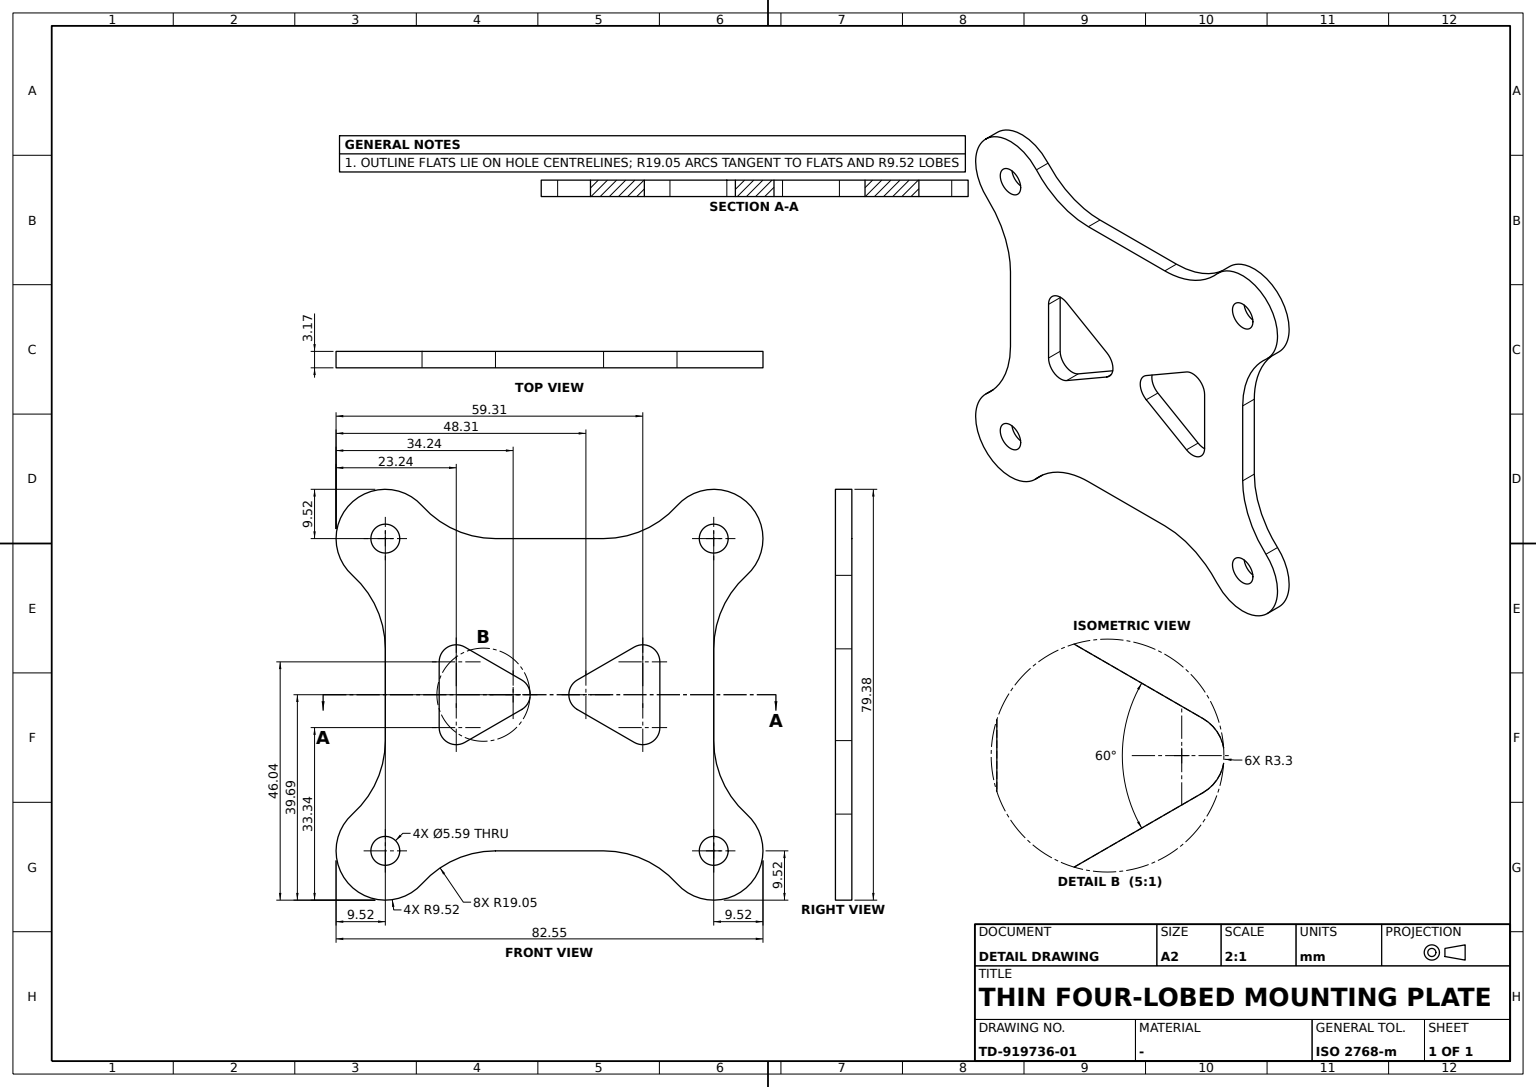
CATIA V5 part; units mm, degrees
sketch "Sketch1" plane through (0, 0, 0) normal (1, 0, 0) x (0, 1, 0)
  line L0 (31.75, 30.1625) -> (31.75, -30.1625)
  line L1 (31.75, -30.1625) -> (-31.75, -30.1625)
  line L2 (-31.75, -30.1625) -> (-31.75, 30.1625)
  line L3 (-31.75, 30.1625) -> (31.75, 30.1625)
  dimension "length L3" = 63.5
  dimension "length L2" = 60.325
  constraint vertical L0 y-axis
  constraint vertical L2 y-axis
  constraint horizontal L1 x-axis
  constraint horizontal L3 x-axis
  constraint equidistance L0 L2 origin
  constraint equidistance L1 L3 origin
extrude "Pad1" add sketch "Sketch1" along normal mid plane 3.175
sketch "Sketch2" plane through (1.5875, 0, 0) normal (1, 0, 0) x (0, 1, 0)
  circle A0 centre (-31.75, 30.1625) radius 9.525
  point P0 (-31.75, 30.1625)
  point P1 (-31.75, 30.1625)
  dimension "radius A0" = 9.525
  constraint coincidence P0 P1
extrude "Pad2" add sketch "Sketch2" against normal blind 3.175
sketch "Sketch3" plane through (1.5875, 0, 0) normal (1, 0, 0) x (0, 1, 0)
  circle A0 centre (-31.75, -30.1625) radius 9.525
  point P0 (-31.75, -30.1625)
  point P1 (-31.75, -30.1625)
  dimension "radius A0" = 9.525
  constraint coincidence P0 P1
extrude "Pad3" add sketch "Sketch3" against normal blind 3.175
sketch "Sketch4" plane through (1.5875, 0, 0) normal (1, 0, 0) x (0, 1, 0)
  circle A0 centre (31.75, 30.1625) radius 9.525
  point P0 (31.75, 30.1625)
  point P1 (31.75, 30.1625)
  dimension "radius A0" = 9.525
  constraint coincidence P0 P1
extrude "Pad4" add sketch "Sketch4" against normal blind 3.175
sketch "Sketch5" plane through (1.5875, 0, 0) normal (1, 0, 0) x (0, 1, 0)
  circle A0 centre (31.75, -30.1625) radius 9.525
  point P0 (31.75, -30.1625)
  point P1 (31.75, -30.1625)
  dimension "radius A0" = 9.525
  constraint coincidence P0 P1
extrude "Pad5" add sketch "Sketch5" against normal blind 3.175
fillet "Fillet1" radius 19.05 1 edges at (0, 31.75, 20.6375)
fillet "Fillet2" radius 19.05 1 edges at (0, 31.75, -20.6375)
fillet "Fillet3" radius 19.05 1 edges at (0, 22.225, 30.1625)
fillet "Fillet4" radius 19.05 1 edges at (0, -22.225, 30.1625)
fillet "Fillet5" radius 19.05 1 edges at (0, -31.75, 20.6375)
fillet "Fillet6" radius 19.05 1 edges at (0, -31.75, -20.6375)
fillet "Fillet7" radius 19.05 1 edges at (0, -22.225, -30.1625)
fillet "Fillet8" radius 19.05 1 edges at (0, 22.225, -30.1625)
sketch "Sketch6" plane through (1.5875, 0, 0) normal (1, 0, 0) x (0, 1, 0)
  circle A0 centre (-31.75, 30.1625) radius 2.794
  circle A1 centre (-31.75, 30.1625) radius 9.525 construction
  dimension "radius A0" = 2.794
  constraint concentricity A0 A1
extrude "Pocket1" cut sketch "Sketch6" against normal up to next
sketch "Sketch7" plane through (1.5875, 0, 0) normal (1, 0, 0) x (0, 1, 0)
  circle A0 centre (31.75, 30.1625) radius 2.794
  circle A1 centre (31.75, 30.1625) radius 9.525 construction
  dimension "radius A0" = 2.794
  constraint concentricity A0 A1
extrude "Pocket2" cut sketch "Sketch7" against normal up to next
sketch "Sketch8" plane through (1.5875, 0, 0) normal (1, 0, 0) x (0, 1, 0)
  circle A0 centre (31.75, -30.1625) radius 2.794
  circle A1 centre (31.75, -30.1625) radius 9.525 construction
  dimension "radius A0" = 2.794
  constraint concentricity A0 A1
extrude "Pocket3" cut sketch "Sketch8" against normal up to next
sketch "Sketch9" plane through (1.5875, 0, 0) normal (1, 0, 0) x (0, 1, 0)
  circle A0 centre (-31.75, -30.1625) radius 2.794
  circle A1 centre (-31.75, -30.1625) radius 9.525 construction
  dimension "radius A0" = 2.794
  constraint concentricity A0 A1
extrude "Pocket4" cut sketch "Sketch9" against normal up to next
sketch "Sketch10" plane through (1.5875, 0, 0) normal (1, 0, 0) x (0, 1, 0)
  line L0 (-21.336, -6.35) -> (-21.336, 6.35)
  point P0 (-21.336, 0)
  point P1 (-21.336, -9.652)
  point P2 (-21.336, 9.652)
  line L1 (-31.75, 30.1625) -> (-31.75, -30.1625) construction
  line L2 (-16.383, 9.2096) -> (-5.3845, 2.8596)
  point P3 (-4.6182, 0)
  line L3 (-16.383, -9.2096) -> (-5.3845, -2.8596)
  arc A0 (-5.3845, 2.8596) -> (-5.3845, -2.8596) centre (-7.0355, 0) cw
  arc A1 (-21.336, 6.35) -> (-16.383, 9.2096) centre (-18.034, 6.35) cw
  point P4 (-18.034, 6.35)
  arc A2 (-16.383, -9.2096) -> (-21.336, -6.35) centre (-18.034, -6.35) cw
  point P5 (-18.034, -6.35)
  dimension "distance L0 L1" = 10.414
  dimension "radius A0" = 3.302
  dimension "radius A1" = 3.302
  dimension "distance P2 P3" = 19.304
  dimension "distance P1 P2" = 19.304
  dimension "length L2" = 12.7
  dimension "distance P4 x axis" = 6.35
  dimension "angle L2 y axis" = 60
  constraint coincidence P0 x-axis
  constraint coincidence P3 x-axis
  constraint coincidence L0 P0
  constraint vertical L0 y-axis
  constraint tangency A0 L2
  constraint tangency A0 L3
  constraint tangency A1 L0
  constraint tangency A1 L2
  constraint tangency A2 L3
  constraint tangency A2 L0
  constraint symmetry P4 P5 x-axis
extrude "Pocket5" cut sketch "Sketch10" against normal up to next
sketch "Sketch11" plane through (1.5875, 0, 0) normal (1, 0, 0) x (0, 1, 0)
  line L0 (21.336, -6.35) -> (21.336, 6.35)
  point P0 (21.336, 0)
  point P1 (21.336, -9.652)
  point P2 (21.336, 9.652)
  line L1 (31.75, -30.1625) -> (31.75, 30.1625) construction
  line L2 (16.383, 9.2096) -> (5.3845, 2.8596)
  point P3 (4.6182, 0)
  line L3 (5.3845, -2.8596) -> (16.383, -9.2096)
  arc A0 (16.383, 9.2096) -> (21.336, 6.35) centre (18.034, 6.35) cw
  point P4 (18.034, 6.35)
  arc A1 (5.3845, 2.8596) -> (5.3845, -2.8596) centre (7.0355, 0) ccw
  arc A2 (16.383, -9.2096) -> (21.336, -6.35) centre (18.034, -6.35) ccw
  point P5 (18.034, -6.35)
  dimension "distance L0 L1" = 10.414
  dimension "radius A0" = 3.302
  dimension "radius A1" = 3.302
  dimension "distance P2 P3" = 19.304
  dimension "distance P1 P2" = 19.304
  dimension "length L2" = 12.7
  dimension "distance P4 x axis" = 6.35
  dimension "angle L2 y axis" = 60
  constraint coincidence P0 x-axis
  constraint coincidence P3 x-axis
  constraint coincidence L0 P0
  constraint vertical L0 y-axis
  constraint tangency A0 L2
  constraint tangency A0 L0
  constraint tangency A1 L2
  constraint tangency A1 L3
  constraint tangency A2 L3
  constraint tangency A2 L0
  constraint symmetry P4 P5 x-axis
extrude "Pocket6" cut sketch "Sketch11" against normal up to next
